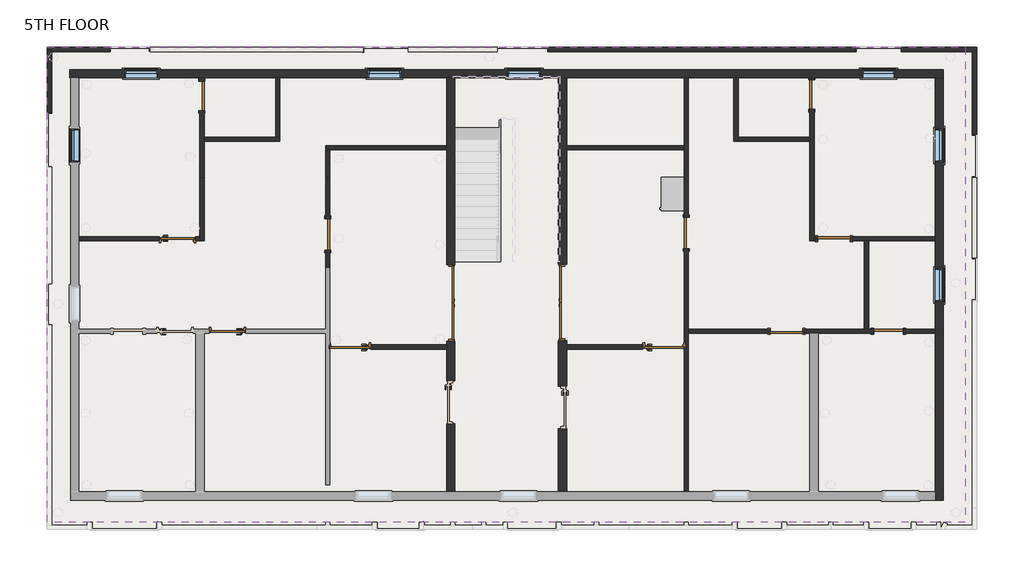
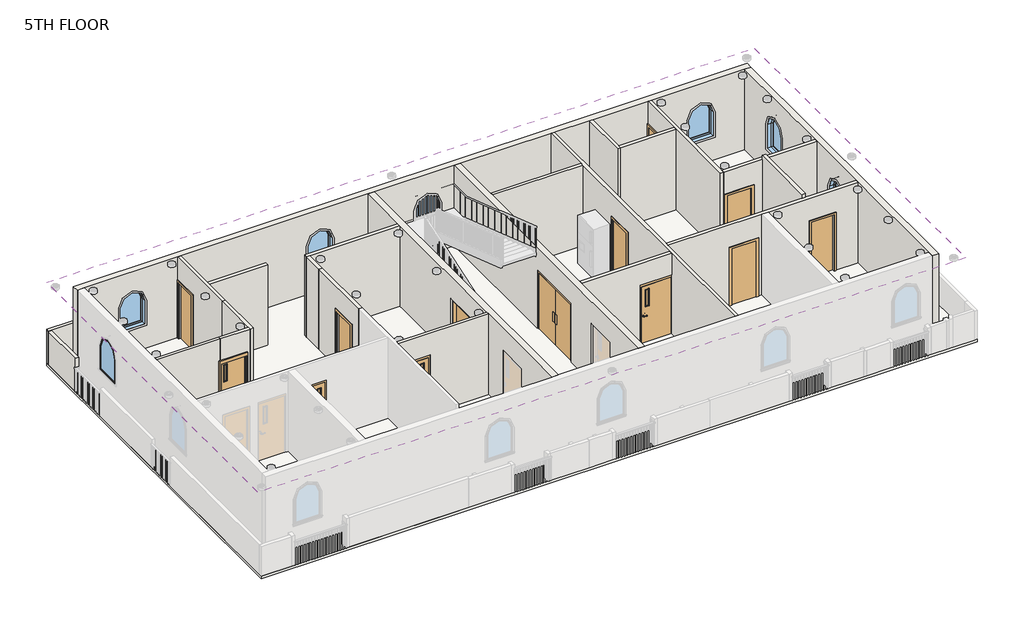
# One storey, part 2 of 7: 32 walls, 13 doors, 7 windows, 2 slabs, 1 covering.
# Revit data of these elements (continued)
# Elements 4, 5 (IfcDoor, "Door-Passage-Single-Vision_Lite : 3'6\"X7' 2") (continued)
#   Rough Height = 7' - 4"
#   Masonry Inset = 0' - 1"
#   MFOpeningWidth = 0' - 4"
#   MFOpeningHeight = 0' - 4"
#   Inset Calculate = 0' - 4"
#   Masonry Frame = yes
#   Dry Wall Frame = no
#   Phase Created = New Construction
#   Materials on its faces: "Metal - Paint Finish - Grey", "Aluminum", "Wood - Birch", "Glass"
# Elements 6, 7 (IfcDoor, "Door-Passage-Single-Vision_Lite : 3'X7'")
#   Swing Angle = 90.00°
#   Rough Width = 3' - 4"
#   Rough Height = 7' - 4"
#   Masonry Inset = 0' - 1"
#   MFOpeningWidth = 0' - 4"
#   MFOpeningHeight = 0' - 4"
#   Inset Calculate = 0' - 4"
#   Masonry Frame = yes
#   Dry Wall Frame = no
#   Phase Created = New Construction
#   Materials on its faces: "Metal - Paint Finish - Grey", "Aluminum", "Wood - Birch", "Glass"
# Elements 8, 9 (IfcDoor, "Single-Flush : 2'10\" x 7'")
#   Phase Created = New Construction
#   Materials on its faces: "Door - Frame", "Door - Panel"
# Elements 10, 11 (IfcDoor, "Single-Flush : 2'11\"x 7'")
#   Phase Created = New Construction
#   Materials on its faces: "Door - Frame", "Door - Panel"
# Elements 12, 13, 14 (IfcDoor, "Single-Flush : 2'8\"x 7'")
#   Phase Created = New Construction
#   Materials on its faces: "Door - Frame", "Door - Panel"
# Elements 15, 16 (IfcSlab, "LW Concrete on Metal Deck")
#   Height Offset From Level = 0' - 0"
#   Phase Created = New Construction
#   Materials on its faces: "Metal Deck", "Concrete, Lightweight"
# Elements 17, 18, 19, 20, 21, 22, 23, 24, 25, 26, 27, 28, 29, 30, 32, 33, 34 (IfcWall, "Generic - 4.5\"")
#   Top Offset = -0' - 6"
#   Base Offset = 0' - 0"
#   wall height = 10' - 0"
#   Phase Created = New Construction
#   Base Constraint = 5TH FLOOR
#   Top Constraint = 6TH FLOOR
#   Materials on its faces: "Default Wall"
# Elements 31, 41 (IfcWall, "Generic - 4.5\"")
#   Top Offset = -6' - 0"
#   Base Offset = 0' - 0"
#   wall height = 4' - 6"
#   Phase Created = New Construction
#   Base Constraint = 5TH FLOOR
#   Top Constraint = 6TH FLOOR
#   Materials on its faces: "Default Wall"
# Element 35 (IfcWall, "Generic - 4.5\"")
#   Top Offset = -6' - 4.43284"
#   Base Offset = 0' - 0"
#   wall height = 4' - 1.56716"
#   Phase Created = New Construction
#   Base Constraint = 5TH FLOOR
#   Top Constraint = 6TH FLOOR
#   Materials on its faces: "Default Wall"
# Element 36 (IfcWall, "Generic - 4.5\"")
#   Top Offset = -6' - 3.86561"
#   Base Offset = 0' - 0"
#   wall height = 4' - 2.13439"
#   Phase Created = New Construction
#   Base Constraint = 5TH FLOOR
#   Top Constraint = 6TH FLOOR
#   Materials on its faces: "Default Wall"
# Element 37 (IfcWall, "Generic - 4.5\"")
#   Top Offset = -6' - 11.32684"
#   Base Offset = 0' - 0"
#   wall height = 3' - 6.67316"
#   Phase Created = New Construction
#   Base Constraint = 5TH FLOOR
#   Top Constraint = 6TH FLOOR
#   Materials on its faces: "Default Wall"
# Element 38 (IfcWall, "Generic - 4.5\"")
#   Top Offset = -6' - 6.91444"
#   Base Offset = 0' - 0"
#   wall height = 3' - 11.08556"
#   Phase Created = New Construction
#   Base Constraint = 5TH FLOOR
#   Top Constraint = 6TH FLOOR
#   Materials on its faces: "Default Wall"
# Element 39 (IfcWall, "Generic - 4.5\"")
#   Top Offset = -6' - 3.83516"
#   Base Offset = 0' - 0"
#   wall height = 4' - 2.16484"
#   Phase Created = New Construction
#   Base Constraint = 5TH FLOOR
#   Top Constraint = 6TH FLOOR
#   Materials on its faces: "Default Wall"
# Element 40 (IfcWall, "Generic - 4.5\"")
#   Top Offset = -6' - 0.2303"
#   Base Offset = 0' - 0"
#   wall height = 4' - 5.7697"
#   Phase Created = New Construction
#   Base Constraint = 5TH FLOOR
#   Top Constraint = 6TH FLOOR
#   Materials on its faces: "Default Wall"
# Element 42 (IfcWall, "Generic - 4.5\"")
#   Top Offset = -6' - 7.02989"
#   Base Offset = 0' - 0"
#   wall height = 3' - 10.97011"
#   Phase Created = New Construction
#   Base Constraint = 5TH FLOOR
#   Top Constraint = 6TH FLOOR
#   Materials on its faces: "Default Wall"
# Elements 43, 44, 45, 46 (IfcWall, "Generic - 9\"")
#   Top Offset = -0' - 6"
#   Base Offset = 0' - 0"
#   wall height = 10' - 0"
#   Phase Created = New Construction
#   Base Constraint = 5TH FLOOR
#   Top Constraint = 6TH FLOOR
#   Materials on its faces: "Concrete Masonry Units"
# Elements 47, 48 (IfcWall, "Interior - 5\" Partition (2-hr)")
#   Top Offset = 0' - 0"
#   Base Offset = 0' - 0"
#   wall height = 10' - 6"
#   Phase Created = New Construction
#   Base Constraint = 5TH FLOOR
#   Top Constraint = 6TH FLOOR
#   Materials on its faces: "Default Wall", "Gypsum Wall Board"
# Element 49 (IfcWindow, "Window-Fixed-Round-Top : 3' x 4'")
#   Mark = "189"
#   Window Inset = 0' - 0"
#   Interior Wall Closure = 0' - 2 1/4"
#   Frame Extension = 0' - 0 1/4"
#   Exterior Wall Closure = 0' - 1 1/4"
#   Interior Trim Visibility = yes
#   Exterior Trim Visibility = yes
#   Phase Created = New Construction
#   Materials on its faces: "Wood - Stained", "Clad - White", "Glass"
# Element 50 (IfcWindow, "Window-Fixed-Round-Top : 3' x 4'")
#   Mark = "190"
#   Window Inset = 0' - 0"
#   Interior Wall Closure = 0' - 2 1/4"
#   Frame Extension = 0' - 0 1/4"
#   Exterior Wall Closure = 0' - 1 1/4"
#   Interior Trim Visibility = yes
#   Exterior Trim Visibility = yes
#   Phase Created = New Construction
#   Materials on its faces: "Wood - Stained", "Clad - White", "Glass"
# Element 51 (IfcWindow, "Window-Fixed-Round-Top : 3' x 4'")
#   Mark = "191"
#   Window Inset = 0' - 0"
#   Interior Wall Closure = 0' - 2 1/4"
#   Frame Extension = 0' - 0 1/4"
#   Exterior Wall Closure = 0' - 1 1/4"
#   Interior Trim Visibility = yes
#   Exterior Trim Visibility = yes
#   Phase Created = New Construction
#   Materials on its faces: "Wood - Stained", "Clad - White", "Glass"
# Element 52 (IfcWindow, "Window-Fixed-Round-Top : 3' x 4'")
#   Mark = "192"
#   Window Inset = 0' - 0"
#   Interior Wall Closure = 0' - 2 1/4"
#   Frame Extension = 0' - 0 1/4"
#   Exterior Wall Closure = 0' - 1 1/4"
#   Interior Trim Visibility = yes
#   Exterior Trim Visibility = yes
#   Phase Created = New Construction
#   Materials on its faces: "Wood - Stained", "Clad - White", "Glass"
# Element 53 (IfcWindow, "Window-Fixed-Round-Top : 3' x 4'")
#   Mark = "193"
#   Window Inset = 0' - 0"
#   Interior Wall Closure = 0' - 2 1/4"
#   Frame Extension = 0' - 0 1/4"
#   Exterior Wall Closure = 0' - 1 1/4"
#   Interior Trim Visibility = yes
#   Exterior Trim Visibility = yes
#   Phase Created = New Construction
#   Materials on its faces: "Wood - Stained", "Clad - White", "Glass"
# Element 54 (IfcWindow, "Window-Fixed-Round-Top : 3' x 4'")
#   Mark = "194"
#   Window Inset = 0' - 0"
#   Interior Wall Closure = 0' - 2 1/4"
#   Frame Extension = 0' - 0 1/4"
#   Exterior Wall Closure = 0' - 1 1/4"
#   Interior Trim Visibility = yes
#   Exterior Trim Visibility = yes
#   Phase Created = New Construction
#   Materials on its faces: "Wood - Stained", "Clad - White", "Glass"
# Element 55 (IfcWindow, "Window-Fixed-Round-Top : 3' x 4'")
#   Mark = "195"
#   Window Inset = 0' - 0"
#   Interior Wall Closure = 0' - 2 1/4"
#   Frame Extension = 0' - 0 1/4"
#   Exterior Wall Closure = 0' - 1 1/4"
#   Interior Trim Visibility = yes
#   Exterior Trim Visibility = yes
#   Phase Created = New Construction
#   Materials on its faces: "Wood - Stained", "Clad - White", "Glass"
# Materials
#   "Default": colour RGB 127 127 127, transparency 0, Cost = 0
#   "Acoustic Ceiling Tile 24 x 48": class "Generic", colour RGB 229 229 229, transparency 0, Description = "Acoustic Ceiling Tile 24 x 48", Cost = 0
#   "Metal - Paint Finish - Brindle": class "Paint", colour RGB 164 133 98, transparency 0, Cost = 0
#   "Metal - Paint Finish - Grey": class "Paint", colour RGB 104 104 104, transparency 0, Cost = 0
#   "Aluminium": class "Metal", colour RGB 244 244 244, transparency 0, Description = "Aluminum 6061", Cost = 0
#   "Wood - Birch": class "Wood", colour RGB 166 116 52, transparency 0, Cost = 0
#   "Glass": class "Glass", colour RGB 0 128 192, transparency 0.75, Description = "Soda Lime Glass", Cost = 0
#   "Aluminum": class "Metal", colour RGB 247 247 247, transparency 0, Description = "Aluminum 6061", Cost = 0
#   "Door - Panel": class "Wood", colour RGB 210 159 95, transparency 0, Cost = 0
#   "Door - Frame": colour RGB 118 70 51, transparency 0, Cost = 0
#   "Concrete, Lightweight": class "Concrete", colour RGB 142 141 140, transparency 0, Description = "Lightweight concrete", Cost = 0
#   "Metal Deck": class "Metal", colour RGB 199 199 199, transparency 0, Description = "Steel, mill finish", Cost = 0
#   "Concrete Masonry Units": class "Masonry", colour RGB 227 227 227, transparency 0, Description = "Concrete masonry units", Cost = 0
#   "Gypsum Wall Board": class "Generic", colour RGB 127 127 127, transparency 0, Description = "Gypsum Wall Board", Cost = 0
#   "Metal Stud Layer": class "Metal", colour RGB 199 199 199, transparency 0, Description = "Light gauge steel framing, thermal air layer", Cost = 0
#   "Wood - Stained": class "Wood", colour RGB 224 178 126, transparency 0, Cost = 0
#   "Clad - White": class "Wood", colour RGB 242 242 238, transparency 0, Cost = 0
#   "Default Wall": colour RGB 128 128 128, transparency 0, Cost = 0
